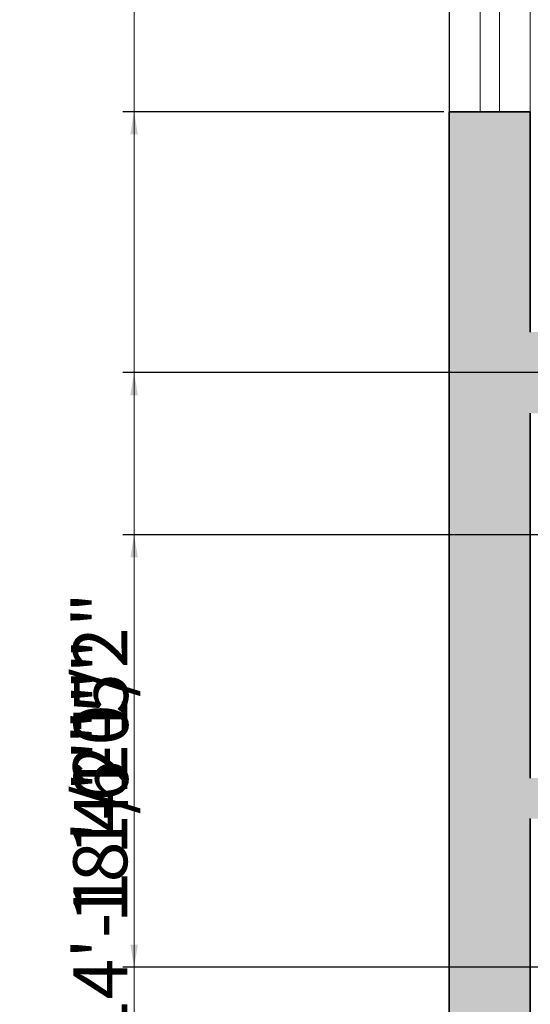
# Model space of a CAD drawing. Units: inches. Extents: x 2696 to 3240, y 1564 to 2310.
# Tile 40 of 76: x 2698 to 2755, y 2071 to 2180. Entities that reach past the tile are written whole.
import ezdxf

# ---------------------------------------------------------------- set-up
doc = ezdxf.new("R2010")
doc.units = ezdxf.units.IN
for name, color, linetype, lineweight in [('A-ANNO-DIMS', 3, 'Continuous', 18), ('A-WALL', 7, 'Continuous', 35), ('A-WALL-PATT', 9, 'Continuous', 13), ('WINDOW', 2, 'Continuous', 18)]:
    doc.layers.add(name, color=color, linetype=linetype, lineweight=lineweight)
doc.styles.add('TIMES NEW', font='times.ttf')
doc.dimstyles.new('Siddhuu', dxfattribs={"dimtxt": 6, "dimasz": 2.5, "dimexe": 1.25, "dimexo": 0.625, "dimtad": 1, "dimdec": 1, "dimlunit": 4, "dimtxsty": 'TIMES NEW', "dimcen": 2.5, "dimclrd": 256, "dimclre": 1, "dimclrt": 7, "dimadec": 0, "dimazin": 0, "dimtfac": 1, "dimtdec": 1, "dimtmove": 0, "dimatfit": 3, "dimfxl": 1, "dimtolj": 1, "dimlwd": -1, "dimarcsym": 0})

# ---------------------------------------------------------------- blocks, each defined once
blk = doc.blocks.new('WD_WIN4')
for p, q in [((-0.5, 0.5), (0.5, 0.5)), ((-0.5, 0.12), (0.5, 0.12)), ((-0.5, -0.12), (0.5, -0.12)), ((-0.5, -0.5), (0.5, -0.5))]:
    blk.add_line(p, q)
blk = doc.blocks.new('*D62')
at = {"layer": 'A-ANNO-DIMS', "color": 1, "lineweight": -2, "transparency": 16777216}
for p, q in [((2965.08, 2140.7), (2709.36, 2140.7)), ((2965.08, 2063.59), (2709.36, 2063.59))]:
    blk.add_line(p, q, dxfattribs=at)
at = {"layer": 'A-ANNO-DIMS', "transparency": 16777216}
blk.add_line((2710.61, 2066.09), (2710.61, 2138.2), dxfattribs=at)
for points in [[(2710.19, 2138.2), (2711.03, 2138.2), (2710.61, 2140.7)], [(2710.19, 2066.09), (2711.03, 2066.09), (2710.61, 2063.59)]]:
    blk.add_solid(points, dxfattribs=at)
at = {"layer": 'Defpoints', "color": 0, "transparency": 16777216}
for p in [(2710.61, 2140.7), (2965.71, 2140.7), (2965.71, 2063.59)]:
    blk.add_point(p, dxfattribs=at)
at = {"layer": 'A-ANNO-DIMS', "color": 7, "transparency": 16777216, "insert": (2706.93, 2102.15), "char_height": 6, "attachment_point": 5, "rotation": 90, "style": 'TIMES NEW'}
blk.add_mtext('\\A1;6\'-5"', dxfattribs=at)
blk = doc.blocks.new('*D64')
at = {"layer": 'A-ANNO-DIMS', "color": 1, "lineweight": -2, "transparency": 16777216}
for p, q in [((3073.08, 2206.7), (2709.36, 2206.7)), ((3068.58, 1989.2), (2709.36, 1989.2))]:
    blk.add_line(p, q, dxfattribs=at)
at = {"layer": 'A-ANNO-DIMS', "transparency": 16777216}
blk.add_line((2710.61, 1991.7), (2710.61, 2204.2), dxfattribs=at)
for points in [[(2710.19, 2204.2), (2711.03, 2204.2), (2710.61, 2206.7)], [(2710.19, 1991.7), (2711.03, 1991.7), (2710.61, 1989.2)]]:
    blk.add_solid(points, dxfattribs=at)
at = {"layer": 'Defpoints', "color": 0, "transparency": 16777216}
for p in [(2710.61, 2206.7), (3073.71, 2206.7), (3069.21, 1989.2)]:
    blk.add_point(p, dxfattribs=at)
at = {"layer": 'A-ANNO-DIMS', "color": 7, "transparency": 16777216, "insert": (2706.85, 2097.95), "char_height": 6, "attachment_point": 5, "rotation": 90, "style": 'TIMES NEW'}
blk.add_mtext('\\A1;18\'-1 1/2"', dxfattribs=at)
blk = doc.blocks.new('*D66')
at = {"layer": 'A-ANNO-DIMS', "color": 1, "lineweight": -2, "transparency": 16777216}
for p, q in [((3077.58, 2122.7), (2709.36, 2122.7)), ((3077.58, 2074.7), (2709.36, 2074.7))]:
    blk.add_line(p, q, dxfattribs=at)
at = {"layer": 'A-ANNO-DIMS', "transparency": 16777216}
blk.add_line((2710.61, 2077.2), (2710.61, 2120.2), dxfattribs=at)
for points in [[(2710.19, 2120.2), (2711.03, 2120.2), (2710.61, 2122.7)], [(2710.19, 2077.2), (2711.03, 2077.2), (2710.61, 2074.7)]]:
    blk.add_solid(points, dxfattribs=at)
at = {"layer": 'Defpoints', "color": 0, "transparency": 16777216}
for p in [(2710.61, 2122.7), (3078.21, 2122.7), (3078.21, 2074.7)]:
    blk.add_point(p, dxfattribs=at)
at = {"layer": 'A-ANNO-DIMS', "color": 7, "transparency": 16777216, "insert": (2706.93, 2098.7), "char_height": 6, "attachment_point": 5, "rotation": 90, "style": 'TIMES NEW'}
blk.add_mtext('\\A1;4\'-0"', dxfattribs=at)
blk = doc.blocks.new('*D68')
at = {"layer": 'A-ANNO-DIMS', "color": 1, "lineweight": -2, "transparency": 16777216}
for p, q in [((2745.61, 2261.58), (2745.61, 1568.95)), ((2782.83, 2261.58), (2782.83, 1568.95))]:
    blk.add_line(p, q, dxfattribs=at)
at = {"layer": 'A-ANNO-DIMS', "transparency": 16777216}
blk.add_line((2748.11, 1570.2), (2780.33, 1570.2), dxfattribs=at)
for points in [[(2748.11, 1570.62), (2748.11, 1569.78), (2745.61, 1570.2)], [(2780.33, 1570.62), (2780.33, 1569.78), (2782.83, 1570.2)]]:
    blk.add_solid(points, dxfattribs=at)
at = {"layer": 'Defpoints', "color": 0, "transparency": 16777216}
for p in [(2745.61, 2262.2), (2782.83, 2262.2), (2782.83, 1570.2)]:
    blk.add_point(p, dxfattribs=at)
at = {"layer": 'A-ANNO-DIMS', "color": 7, "transparency": 16777216, "insert": (2764.22, 1573.88), "char_height": 6, "attachment_point": 5, "style": 'TIMES NEW'}
blk.add_mtext('\\A1;3\'-1"', dxfattribs=at)
blk = doc.blocks.new('*D72')
at = {"layer": 'A-ANNO-DIMS', "color": 1, "lineweight": -2, "transparency": 16777216}
for p, q in [((2744.99, 2169.67), (2709.36, 2169.67)), ((2744.99, 2000.2), (2709.36, 2000.2))]:
    blk.add_line(p, q, dxfattribs=at)
at = {"layer": 'A-ANNO-DIMS', "transparency": 16777216}
blk.add_line((2710.61, 2167.17), (2710.61, 2002.7), dxfattribs=at)
for points in [[(2710.19, 2167.17), (2711.03, 2167.17), (2710.61, 2169.67)], [(2710.19, 2002.7), (2711.03, 2002.7), (2710.61, 2000.2)]]:
    blk.add_solid(points, dxfattribs=at)
at = {"layer": 'Defpoints', "color": 0, "transparency": 16777216}
for p in [(2745.61, 2169.67), (2710.61, 2000.2), (2745.61, 2000.2)]:
    blk.add_point(p, dxfattribs=at)
at = {"layer": 'A-ANNO-DIMS', "color": 7, "transparency": 16777216, "insert": (2706.85, 2084.94), "char_height": 6, "attachment_point": 5, "rotation": 90, "style": 'TIMES NEW'}
blk.add_mtext('\\A1;14\'-1 1/2"', dxfattribs=at)

msp = doc.modelspace()

# ---------------------------------------------------------------- hatches: boundary and pattern name
at = {"layer": 'A-WALL-PATT', "transparency": 33554556}
h = msp.add_hatch(color=256, dxfattribs=at)
h.dxf.hatch_style = 1
h.paths.add_polyline_path([(2879.11, 2253.2), (2905.91, 2253.2), (2905.91, 2262.2), (2841.89, 2262.2), (2841.89, 2253.2), (2870.11, 2253.2), (2870.11, 2176.6), (2965.71, 2176.6), (2965.71, 2206.7), (2973.58, 2206.7), (2973.58, 2215.7), (2965.71, 2215.7), (2965.71, 2262.2), (2929.91, 2262.2), (2929.91, 2253.2), (2956.71, 2253.2), (2956.71, 2185.6), (2879.11, 2185.6)])
h.paths.add_polyline_path([(2782.83, 2262.2), (2745.61, 2262.2), (2745.61, 2228.73), (2754.61, 2228.73), (2754.61, 2253.2), (2782.83, 2253.2)])
h.paths.add_polyline_path([(2754.61, 2136.2), (2965.71, 2136.2), (2965.71, 2145.2), (2879.11, 2145.2), (2879.11, 2147.07), (2877.34, 2147.07), (2870.11, 2147.07), (2870.11, 2145.2), (2754.61, 2145.2), (2754.61, 2169.67), (2745.61, 2169.67), (2745.61, 2000.2), (2754.61, 2000.2), (2754.61, 2019.2), (2849.08, 2019.2), (2849.08, 2023.7), (2841.21, 2023.7), (2841.21, 2051.83), (2836.71, 2051.83), (2836.71, 2023.7), (2754.61, 2023.7), (2754.61, 2091.2), (2836.71, 2091.2), (2836.71, 2087.83), (2841.21, 2087.83), (2841.21, 2095.7), (2754.61, 2095.7)])
h.paths.add_polyline_path([(2965.71, 2136.2), (2956.71, 2136.2), (2956.71, 2023.7), (2885.08, 2023.7), (2885.08, 2019.2), (2956.71, 2019.2), (2956.71, 1950.58), (2965.71, 1950.58), (2965.71, 1980.2), (2973.58, 1980.2), (2973.58, 1989.2), (2965.71, 1989.2)])
h.paths.add_polyline_path([(2754.61, 1906.7), (2880.21, 1906.7), (2884.71, 1906.7), (2956.71, 1906.7), (2956.71, 1792.7), (2944.71, 1792.7), (2944.71, 1783.7), (2956.71, 1783.7), (2956.71, 1740.2), (2884.71, 1740.2), (2884.71, 1783.7), (2896.71, 1783.7), (2896.71, 1792.7), (2884.71, 1792.7), (2884.71, 1846.7), (2880.21, 1846.7), (2880.21, 1740.2), (2754.61, 1740.2), (2754.61, 1777.2), (2745.61, 1777.2), (2745.61, 1692.7), (2754.61, 1692.7), (2754.61, 1731.2), (2956.71, 1731.2), (2956.71, 1723.33), (2965.71, 1723.33), (2965.71, 1884.2), (2973.58, 1884.2), (2973.58, 1893.2), (2965.71, 1893.2), (2965.71, 1914.58), (2956.71, 1914.58), (2956.71, 1911.2), (2754.61, 1911.2), (2754.61, 1930.2), (2745.61, 1930.2), (2745.61, 1817.2), (2754.61, 1817.2), (2754.61, 1854.2), (2826.61, 1854.2), (2826.61, 1868.83), (2822.11, 1868.83), (2822.11, 1858.7), (2754.61, 1858.7)])
h.paths.add_polyline_path([(2965.71, 1656.2), (3008.24, 1656.2), (3008.24, 1665.2), (2965.71, 1665.2), (2965.71, 1693.33), (2956.71, 1693.33), (2956.71, 1686.2), (2934.58, 1686.2), (2934.58, 1681.7), (2956.71, 1681.7), (2956.71, 1614.2), (2896.71, 1614.2), (2896.71, 1681.7), (2904.58, 1681.7), (2904.58, 1686.2), (2892.21, 1686.2), (2892.21, 1614.2), (2858.41, 1614.2), (2858.41, 1605.2), (2965.71, 1605.2)])
h.paths.add_polyline_path([(2788.41, 1614.2), (2754.61, 1614.2), (2754.61, 1652.7), (2745.61, 1652.7), (2745.61, 1605.2), (2788.41, 1605.2)])
h.paths.add_polyline_path([(3199.61, 1633.05), (3190.61, 1633.05), (3190.61, 1614.2), (3082.61, 1614.2), (3082.61, 1665.2), (3070.24, 1665.2), (3070.24, 1656.2), (3078.11, 1656.2), (3078.11, 1605.2), (3199.61, 1605.2)])
h.paths.add_polyline_path([(3199.61, 1702.05), (3190.61, 1702.05), (3190.61, 1699.7), (3106.61, 1699.7), (3106.61, 1747.7), (3190.61, 1747.7), (3190.61, 1752.2), (3082.61, 1752.2), (3082.61, 1760.08), (3078.11, 1760.08), (3078.11, 1747.7), (3102.11, 1747.7), (3102.11, 1699.7), (3078.11, 1699.7), (3078.11, 1695.2), (3190.61, 1695.2), (3190.61, 1676.35), (3199.61, 1676.35)])
h.paths.add_polyline_path([(3199.61, 1783.2), (3190.61, 1783.2), (3190.61, 1745.35), (3199.61, 1745.35)])
h.paths.add_polyline_path([(3082.61, 1884.2), (3190.61, 1884.2), (3190.61, 1853.2), (3199.61, 1853.2), (3199.61, 1901.7), (3190.61, 1901.7), (3190.61, 1893.2), (3005.58, 1893.2), (3005.58, 1891.28), (3005.58, 1884.2), (3078.11, 1884.2), (3078.11, 1792.08), (3082.61, 1792.08)])
h.paths.add_polyline_path([(3199.61, 1994.7), (3190.61, 1994.7), (3190.61, 1989.2), (3073.71, 1989.2), (3073.71, 2034.2), (3069.21, 2034.2), (3069.21, 1989.2), (3005.58, 1989.2), (3005.58, 1980.2), (3190.61, 1980.2), (3190.61, 1971.7), (3199.61, 1971.7)])
h.paths.add_polyline_path([(3199.61, 2155.2), (3190.61, 2155.2), (3190.61, 2064.7), (3199.61, 2064.7)])
h.paths.add_polyline_path([(3190.61, 2074.7), (3106.61, 2074.7), (3106.61, 2122.7), (3190.61, 2122.7), (3190.61, 2127.2), (3082.71, 2127.2), (3082.71, 2135.08), (3073.71, 2135.08), (3073.71, 2122.7), (3102.11, 2122.7), (3102.11, 2074.7), (3069.21, 2074.7), (3069.21, 2070.2), (3190.61, 2070.2)])
h.paths.add_polyline_path([(3082.71, 2253.2), (3190.61, 2253.2), (3190.61, 2225.2), (3199.61, 2225.2), (3199.61, 2262.2), (3073.71, 2262.2), (3073.71, 2215.7), (3035.58, 2215.7), (3035.58, 2206.7), (3073.71, 2206.7), (3073.71, 2171.08), (3082.71, 2171.08)])

# ---------------------------------------------------------------- linework, layer by layer
at = {"layer": 'A-WALL'}
for p, q in [((2754.61, 2169.67), (2745.61, 2169.67)), ((2745.61, 2000.2), (2745.61, 2169.67)), ((2754.61, 2145.2), (2754.61, 2169.67)), ((2754.61, 2095.7), (2754.61, 2136.2)), ((2754.61, 2023.7), (2754.61, 2091.2))]:
    msp.add_line(p, q, dxfattribs=at)

# ---------------------------------------------------------------- block references
at = {"layer": 'WINDOW', "xscale": 59.05511811023622, "yscale": 8.999999999999545, "zscale": 59.05511811023622, "rotation": 269.9999999999996}
msp.add_blockref('WD_WIN4', (2750.11, 2199.2), dxfattribs=at)

# ---------------------------------------------------------------- dimensions: what is measured, and where the dimension line sits
at = {"layer": 'A-ANNO-DIMS'}
dim = msp.add_linear_dim(base=(2782.83, 1570.2), p1=(2745.61, 2262.2), p2=(2782.83, 2262.2), dimstyle='Siddhuu', override={"dimdec": 1, "dimlfac": 1, "dimrnd": 0, "dimzin": 1, "dimdsep": 46, "dimlunit": 4, "dimfrac": 2}, dxfattribs=at)
dim.commit()
dim.dimension.update_dxf_attribs({"geometry": '*D68', "text_midpoint": (2764.22, 1573.88)})
for base, p1, p2, picture, middle in [((2710.61, 2206.7), (3069.21, 1989.2), (3073.71, 2206.7), '*D64', (2706.85, 2097.95)), ((2710.61, 2000.2), (2745.61, 2169.67), (2745.61, 2000.2), '*D72', (2706.85, 2084.94)), ((2710.61, 2140.7), (2965.71, 2063.59), (2965.71, 2140.7), '*D62', (2706.93, 2102.15)), ((2710.61, 2122.7), (3078.21, 2074.7), (3078.21, 2122.7), '*D66', (2706.93, 2098.7))]:
    dim = msp.add_linear_dim(base=base, p1=p1, p2=p2, angle=90, dimstyle='Siddhuu', override={"dimdec": 1, "dimlfac": 1, "dimrnd": 0, "dimzin": 1, "dimdsep": 46, "dimlunit": 4, "dimfrac": 2}, dxfattribs=at)
    dim.commit()
    dim.dimension.update_dxf_attribs({"geometry": picture, "text_midpoint": middle})

doc.saveas('drawing.dxf')
